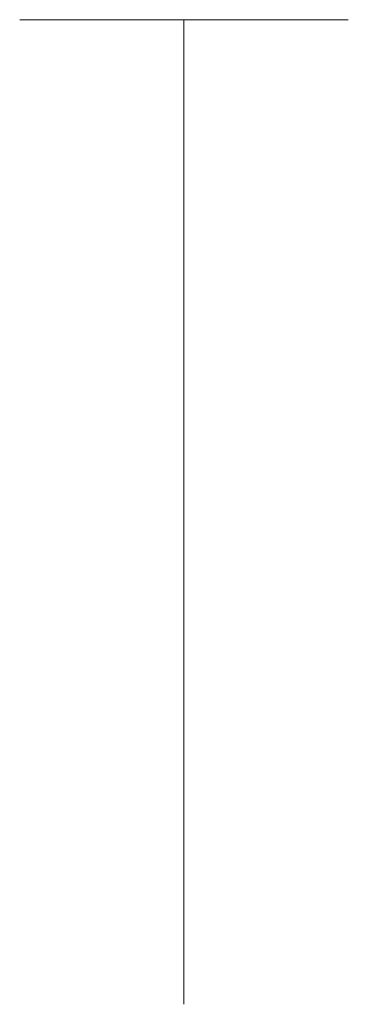
# Model space of a CAD drawing. Units: millimetres. Extents: x 168.7 to 182.7, y 261.3 to 303.3.
import ezdxf

# ---------------------------------------------------------------- set-up
doc = ezdxf.new("R2010")
doc.units = ezdxf.units.MM
doc.layers.add('M-CONS', color=8, linetype='Continuous', lineweight=13)

msp = doc.modelspace()

# ---------------------------------------------------------------- linework, layer by layer
at = {"layer": 'M-CONS'}
for p, q in [((168.677, 303.287, 20), (182.677, 303.287, 20)), ((175.677, 303.287, 20), (175.677, 261.287, 20))]:
    msp.add_line(p, q, dxfattribs=at)

doc.saveas('drawing.dxf')
